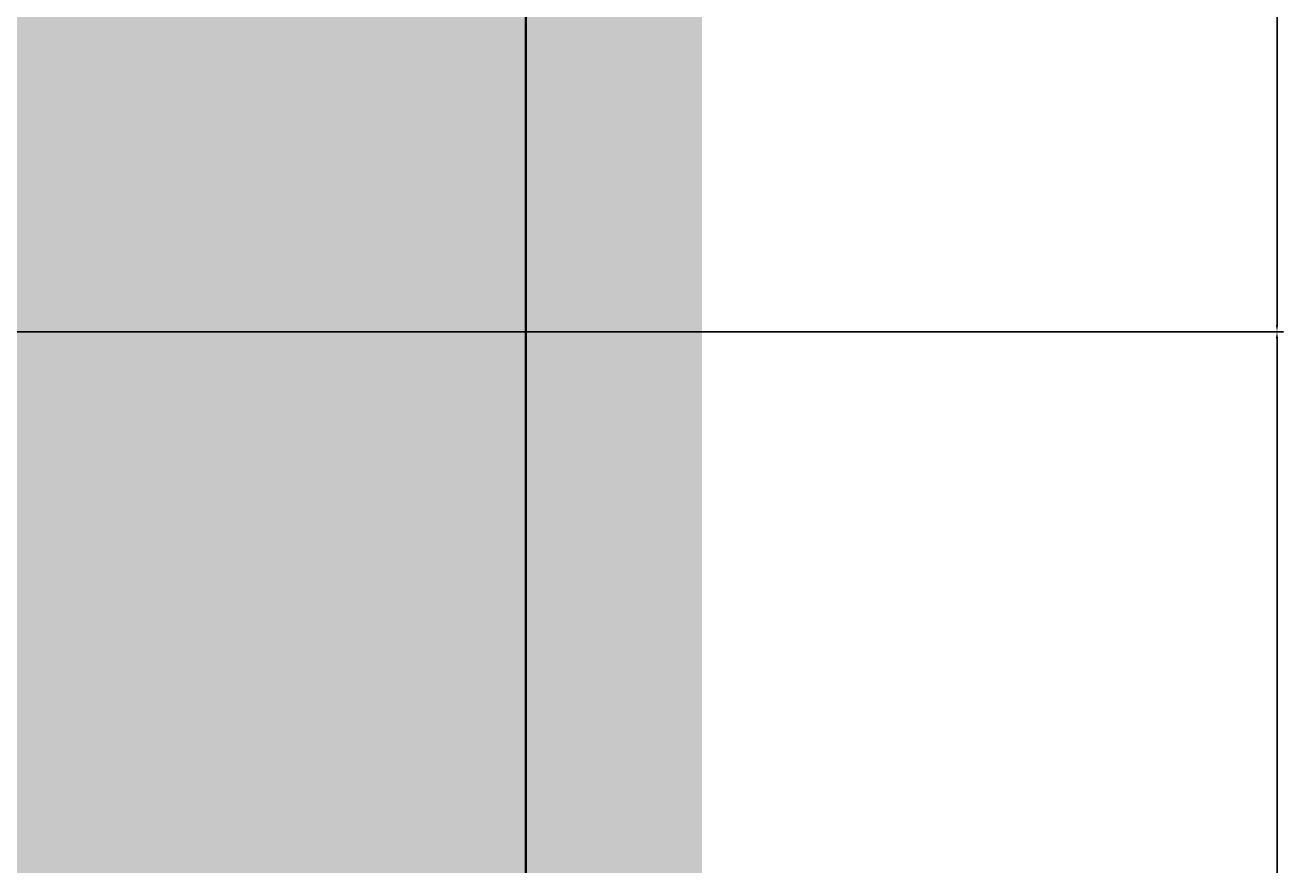
# Model space of a CAD drawing. Units: feet. Extents: x 2695 to 2912, y 795 to 1139.
# Tile 33 of 83: x 2877 to 2912, y 891 to 914. Entities that reach past the tile are written whole.
import ezdxf

# ---------------------------------------------------------------- set-up
doc = ezdxf.new("R2010")
doc.units = ezdxf.units.FT
for name, color, linetype, lineweight in [('A-ANNO-DIMS', 2, 'Continuous', 18), ('A-ELEV', 7, 'Continuous', 35), ('A-ELEV-PATT', 252, 'Continuous', 13)]:
    doc.layers.add(name, color=color, linetype=linetype, lineweight=lineweight)
doc.styles.get("Standard").update_dxf_attribs({"font": 'arial.ttf'})
doc.dimstyles.get("Standard").update_dxf_attribs({"dimtxt": 0.18, "dimasz": 0.18, "dimexe": 0.18, "dimexo": 0.0625, "dimgap": 0.09, "dimtad": 0, "dimtih": 1, "dimtoh": 1, "dimdec": 1, "dimzin": 0, "dimdsep": 46, "dimlunit": 3, "dimtxsty": 'Standard', "dimcen": 0.09, "dimadec": 0, "dimazin": 0, "dimtfac": 1, "dimtdec": 1, "dimtofl": 0, "dimtmove": 0, "dimatfit": 3, "dimfxl": 1, "dimtolj": 1, "dimtzin": 0, "dimarcsym": 0})

# ---------------------------------------------------------------- blocks, each defined once
blk = doc.blocks.new('*D14')
at = {"layer": 'A-ANNO-DIMS', "color": 0, "lineweight": -2, "transparency": 16777216}
for p, q in [((2838.439, 905.514), (2911.424, 905.514)), ((2911.244, 905.334), (2911.244, 890.368)), ((2911.244, 875.037), (2911.244, 890.004)), ((2758.214, 874.857), (2911.424, 874.857))]:
    blk.add_line(p, q, dxfattribs=at)
at = {"layer": 'A-ANNO-DIMS', "color": 0, "transparency": 16777216}
for points in [[(2911.214, 905.334), (2911.274, 905.334), (2911.244, 905.514)], [(2911.214, 875.037), (2911.274, 875.037), (2911.244, 874.857)]]:
    blk.add_solid(points, dxfattribs=at)
at = {"layer": 'Defpoints', "color": 0, "transparency": 16777216}
for p in [(2838.377, 905.514), (2911.244, 905.514), (2758.151, 874.857)]:
    blk.add_point(p, dxfattribs=at)
at = {"layer": 'A-ANNO-DIMS', "color": 0, "transparency": 16777216, "insert": (2911.244, 890.186), "char_height": 0.18, "attachment_point": 5}
blk.add_mtext('\\A1;30.66', dxfattribs=at)
blk = doc.blocks.new('*D15')
at = {"layer": 'A-ANNO-DIMS', "color": 0, "lineweight": -2, "transparency": 16777216}
for p, q in [((2890.699, 924.311), (2911.424, 924.311)), ((2911.244, 924.131), (2911.244, 915.094)), ((2911.244, 905.694), (2911.244, 914.731)), ((2838.439, 905.514), (2911.424, 905.514))]:
    blk.add_line(p, q, dxfattribs=at)
at = {"layer": 'A-ANNO-DIMS', "color": 0, "transparency": 16777216}
for points in [[(2911.214, 924.131), (2911.274, 924.131), (2911.244, 924.311)], [(2911.214, 905.694), (2911.274, 905.694), (2911.244, 905.514)]]:
    blk.add_solid(points, dxfattribs=at)
at = {"layer": 'Defpoints', "color": 0, "transparency": 16777216}
for p in [(2890.636, 924.311), (2911.244, 924.311), (2838.377, 905.514)]:
    blk.add_point(p, dxfattribs=at)
at = {"layer": 'A-ANNO-DIMS', "color": 0, "transparency": 16777216, "insert": (2911.244, 914.912), "char_height": 0.18, "attachment_point": 5}
blk.add_mtext('\\A1;18.796', dxfattribs=at)

msp = doc.modelspace()

# ---------------------------------------------------------------- hatches: boundary and pattern name
at = {"layer": 'A-ELEV-PATT'}
h = msp.add_hatch(color=256, dxfattribs=at)
h.set_gradient(color1=(147, 149, 152), color2=(147, 149, 152), tint=1)
h.paths.add_polyline_path([(2770.6361, 1118.4096), (2710.6361, 1118.4096), (2710.6361, 1062.9306), (2770.6361, 1062.9306)])
h.paths.add_polyline_path([(2890.6361, 1103.3378), (2770.6361, 1103.3378), (2770.6361, 1062.9306), (2890.6361, 1062.9306)])
h.paths.add_polyline_path([(2730.7081, 1048.1052), (2755.1125, 1048.1052), (2755.1125, 936.9306), (2770.6361, 936.9306), (2770.6361, 1050.3105), (2715.8852, 1050.3105), (2715.8852, 936.9306), (2730.7081, 936.9306)])
h.paths.add_polyline_path([(2890.6361, 1050.3105), (2770.6361, 1050.3105), (2770.6361, 971.9673), (2778.0341, 971.9673), (2778.0341, 1020.8235), (2843.575, 1020.8235), (2843.575, 971.9673), (2890.6361, 971.9673)])
h.paths.add_polyline_path([(2888.1882, 970.7156), (2843.575, 970.7156), (2843.575, 964.8267), (2888.1882, 964.8267)])
h.paths.add_polyline_path([(2888.1882, 964.1328), (2843.575, 964.1328), (2843.575, 956.614), (2888.1882, 956.614)])
h.paths.add_polyline_path([(2888.1882, 955.9202), (2843.575, 955.9202), (2843.575, 949.2892), (2888.1882, 949.2892)])
h.paths.add_polyline_path([(2888.1882, 948.5954), (2843.575, 948.5954), (2843.575, 941.3507), (2888.1882, 941.3507)])
h.paths.add_polyline_path([(2888.1882, 940.6569), (2843.575, 940.6569), (2843.575, 936.9306), (2888.1882, 936.9306)])
h.paths.add_polyline_path([(2890.6361, 970.7156), (2888.9368, 970.7156), (2888.9368, 964.8267), (2890.6361, 964.8267)])
h.paths.add_polyline_path([(2890.6361, 964.1328), (2888.9368, 964.1328), (2888.9368, 956.614), (2890.6361, 956.614)])
h.paths.add_polyline_path([(2890.6361, 955.9202), (2888.9368, 955.9202), (2888.9368, 949.2892), (2890.6361, 949.2892)])
h.paths.add_polyline_path([(2890.6361, 940.6569), (2888.9368, 940.6569), (2888.9368, 936.9306), (2890.6361, 936.9306)])
h.paths.add_polyline_path([(2890.6361, 948.5954), (2888.9368, 948.5954), (2888.9368, 941.3507), (2890.6361, 941.3507)])
h.paths.add_polyline_path([(2772.5216, 970.7156), (2770.6361, 970.7156), (2770.6361, 964.8267), (2772.5216, 964.8267)])
h.paths.add_polyline_path([(2772.5216, 964.1328), (2770.6361, 964.1328), (2770.6361, 956.614), (2772.5216, 956.614)])
h.paths.add_polyline_path([(2772.5216, 955.9202), (2770.6361, 955.9202), (2770.6361, 949.2892), (2772.5216, 949.2892)])
h.paths.add_polyline_path([(2772.5216, 948.5954), (2770.6361, 948.5954), (2770.6361, 941.3507), (2772.5216, 941.3507)])
h.paths.add_polyline_path([(2772.5216, 940.6569), (2770.6361, 940.6569), (2770.6361, 936.9306), (2772.5216, 936.9306)])
h.paths.add_polyline_path([(2778.0341, 940.6569), (2773.2702, 940.6569), (2773.2702, 936.9306), (2778.0341, 936.9306)])
h.paths.add_polyline_path([(2778.0341, 970.7156), (2773.2702, 970.7156), (2773.2702, 964.8267), (2778.0341, 964.8267)])
h.paths.add_polyline_path([(2778.0341, 964.1328), (2773.2702, 964.1328), (2773.2702, 956.614), (2778.0341, 956.614)])
h.paths.add_polyline_path([(2778.0341, 955.9202), (2773.2702, 955.9202), (2773.2702, 949.2892), (2778.0341, 949.2892)])
h.paths.add_polyline_path([(2778.0341, 948.5954), (2773.2702, 948.5954), (2773.2702, 941.3507), (2778.0341, 941.3507)])
h.paths.add_polyline_path([(2810.0407, 940.6569), (2780.0341, 940.6569), (2780.0341, 936.9306), (2810.0407, 936.9306)])
h.paths.add_polyline_path([(2890.6361, 924.3105), (2770.6361, 924.3105), (2770.6361, 810.9306), (2773.5029, 810.9306), (2773.5029, 905.5143), (2805.9398, 905.5143), (2838.3767, 905.5143), (2838.3767, 810.9306), (2890.6361, 810.9306)])
h = msp.add_hatch(color=256, dxfattribs=at)
h.set_gradient(color1=(255, 255, 255), tint=1)
h.paths.add_polyline_path([(2895.4694, 1107.8588), (2890.6361, 1107.8588), (2890.6361, 810.9306), (2895.4694, 810.9306)])

# ---------------------------------------------------------------- linework, layer by layer
at = {"layer": 'A-ELEV'}
for p, q in [((2890.6361, 810.9306), (2890.6361, 1107.8588)), ((2890.6361, 1062.9306), (2890.6361, 810.9306))]:
    msp.add_line(p, q, dxfattribs=at)

# ---------------------------------------------------------------- dimensions: what is measured, and where the dimension line sits
at = {"layer": 'A-ANNO-DIMS'}
for base, p1, p2, override, picture, middle in [((2911.2444, 924.3105), (2838.3767, 905.5143), (2890.6361, 924.3105), {"dimdec": 3, "dimlfac": 1, "dimrnd": 0, "dimzin": 0, "dimdsep": 46, "dimlunit": 2}, '*D15', (2911.2444, 914.9124)), ((2911.2444, 905.5143), (2758.1515, 874.8571), (2838.3767, 905.5143), {"dimdec": 2, "dimlfac": 1, "dimrnd": 0, "dimzin": 0, "dimdsep": 46, "dimlunit": 2}, '*D14', (2911.2444, 890.1857))]:
    dim = msp.add_linear_dim(base=base, p1=p1, p2=p2, angle=90, dimstyle='Standard', override=override, dxfattribs=at)
    dim.commit()
    dim.dimension.update_dxf_attribs({"geometry": picture, "text_midpoint": middle})

doc.saveas('drawing.dxf')
